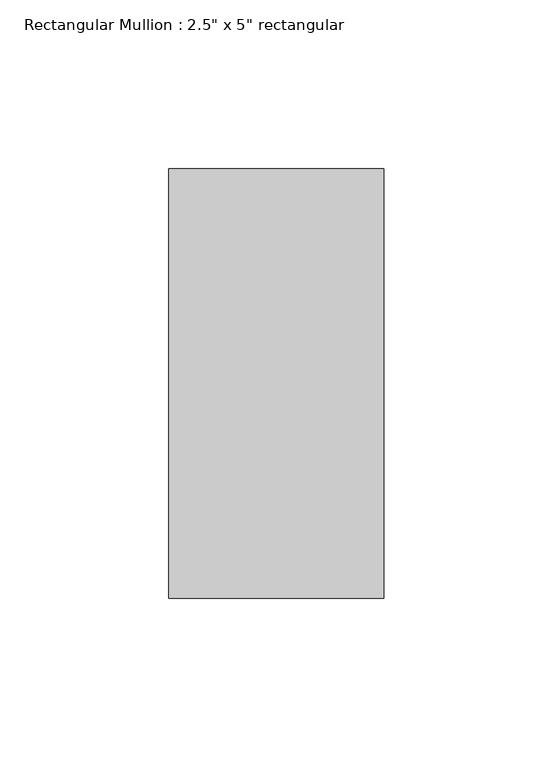
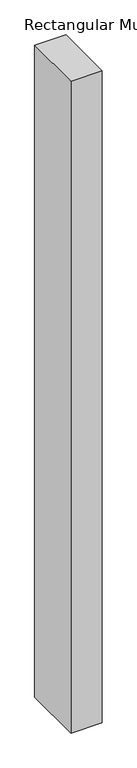
"""IFC4 building model written with IfcOpenShell, lengths in millimetres: member geometry."""

from ifc_helpers import new_model, si_unit, frame, origin, place, context, project, spatial, polyline, outline, extrude, source, transform, mapped, element, save


def member_c646c215(model_context):
    return source(origin(), model_context, "Body", "SweptSolid", [
        extrude(outline(polyline([(0.0, 63.5), (0.0, -63.5), (-63.5, -63.5), (-63.5, 63.5), (0.0, 63.5)])), frame((0.0, 0.0, -1398.2371896), z_axis=(0.0, 0.0, 1.0), x_axis=(1.0, 0.0, 0.0)), (0.0, 0.0, 1.0), 1398.2371896),
    ])


if __name__ == "__main__":
    model = new_model("IFC4")
    model_context = context("Model", 3, world=origin())
    ifc_project = project(units=[si_unit("LENGTHUNIT", "METRE", prefix="MILLI")], contexts=[model_context])
    site = spatial("IfcSite", under=ifc_project)
    building = spatial("IfcBuilding", under=site)
    placement = place(None, origin())
    member_shape = member_c646c215(model_context)
    element("IfcMember", 1, ObjectType="Rectangular Mullion : 2.5\" x 5\" rectangular", at=placement, inside=building, context=model_context, shape_type="MappedRepresentation", body=[
        mapped(member_shape, transform((0.0, 0.0, 0.0), x_axis=(1.0, 0.0, 0.0), y_axis=(0.0, 1.0, 0.0), z_axis=(0.0, 0.0, 1.0))),
    ])
    save(model, "model.ifc")

# Revit data of these elements
# Type "Rectangular Mullion : 2.5\" x 5\" rectangular"
#   built-in parameter 1007304 = 0.416667 (stored number, unit not read)
#   built-in parameter 1007301 = 0.104167 (stored number, unit not read)
#   built-in parameter 1007300 = 0.104167 (stored number, unit not read)
# Element 1 (IfcMember, "Rectangular Mullion : 2.5\" x 5\" rectangular")
#   Materials on its faces: "Aluminum"
# Materials
#   "Aluminum": class "Metal", colour RGB 247 247 247, transparency 0, Description = "Aluminum 6061", Cost = 0
